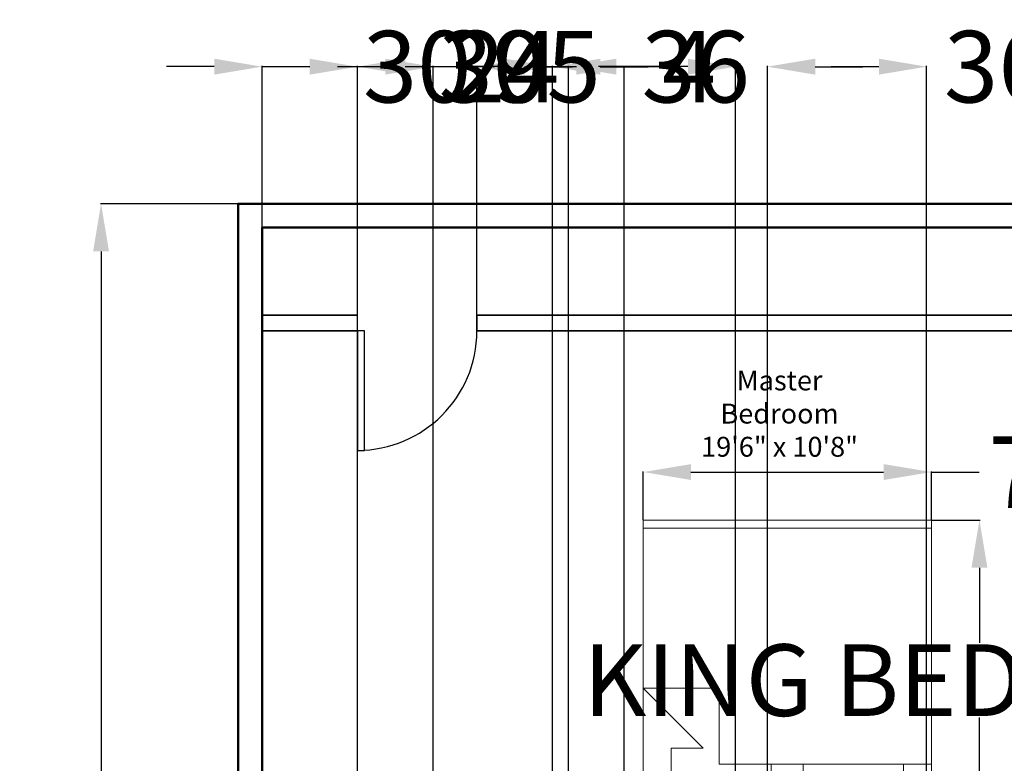
# Model space of a CAD drawing. Units: inches. Extents: x -230 to 384, y -962 to -183.
# Tile 5 of 6: x -156 to 91, y -370 to -183. Entities that reach past the tile are written whole.
import ezdxf

# ---------------------------------------------------------------- set-up
doc = ezdxf.new("R2010")
doc.units = ezdxf.units.IN
for name, color, linetype, lineweight in [('A-ANNO-DIMS', 2, 'Continuous', 18), ('A-AREA-IDEN', 7, 'Continuous', 18), ('A-DOOR', 3, 'Continuous', 25), ('Furniture', 2, 'Continuous', 18), ('Inner Wall', 5, 'Continuous', 35), ('Outer Wall', 1, 'Continuous', 50)]:
    doc.layers.add(name, color=color, linetype=linetype, lineweight=lineweight)
doc.styles.get("Standard").update_dxf_attribs({"font": 'arial.ttf'})
doc.dimstyles.get("Standard").update_dxf_attribs({"dimtxt": 18, "dimasz": 12, "dimexe": 0.18, "dimexo": 0.0625, "dimgap": 0.09, "dimtad": 0, "dimtih": 1, "dimtoh": 1, "dimdec": 0, "dimzin": 0, "dimdsep": 46, "dimlunit": 3, "dimtxsty": 'Standard', "dimcen": 0.09, "dimadec": 0, "dimazin": 0, "dimtfac": 1, "dimtdec": 0, "dimtofl": 0, "dimtmove": 0, "dimatfit": 3, "dimfxl": 1, "dimtolj": 1, "dimtzin": 0, "dimarcsym": 0})

# ---------------------------------------------------------------- blocks, each defined once
blk = doc.blocks.new('*U3')
for p, q in [((-30, 0), (-30, -4)), ((0, 0), (0, -4))]:
    blk.add_line(p, q)
blk.add_lwpolyline([(0, 0), (0, 30), (-1.75, 30), (-1.75, 0)], close=True)
blk.add_arc((0, 0), 30, 90, 180)
blk = doc.blocks.new('KING-00')
for p, q in [((-0.8967, -0.947), (-0.8967, 0.8818)), ((0.6019, 0.8818), (0.6019, -0.4644)), ((1.0337, -0.947), (1.0337, 0.8818)), ((0.6019, 0.704), (0.8813, 0.704)), ((0.8813, 0.069), (0.8813, 0.704)), ((0.6019, 0.069), (0.8813, 0.069)), ((0.8813, -0.1342), (0.6019, -0.1342)), ((0.8813, -0.7692), (0.8813, -0.1342)), ((0.1193, -0.4644), (0.1193, -0.947)), ((0.6019, -0.4644), (0.1193, -0.4644)), ((0.1193, -0.947), (0.5003, -0.566)), ((0.5003, -0.7692), (0.5003, -0.566)), ((0.5003, -0.7692), (0.8813, -0.7692))]:
    blk.add_line(p, q)
blk.add_lwpolyline([(-0.9475, -0.947), (-0.9475, 0.8818), (1.0845, 0.8818), (1.0845, -0.947)], close=True)
blk = doc.blocks.new('*D16')
at = {"layer": 'A-ANNO-DIMS', "color": 0, "lineweight": -2, "transparency": 16777216}
for p, q in [((72.67, -308.78), (84.86, -308.78)), ((84.68, -320.78), (84.68, -339.62)), ((84.68, -377.25), (84.68, -358.42)), ((72.67, -389.25), (84.86, -389.25))]:
    blk.add_line(p, q, dxfattribs=at)
at = {"layer": 'A-ANNO-DIMS', "color": 0, "transparency": 16777216}
for points in [[(82.68, -320.78), (86.68, -320.78), (84.68, -308.78)], [(82.68, -377.25), (86.68, -377.25), (84.68, -389.25)]]:
    blk.add_solid(points, dxfattribs=at)
at = {"layer": 'Defpoints', "color": 0, "transparency": 16777216}
for p in [(72.61, -308.78), (72.61, -389.25), (84.68, -389.25)]:
    blk.add_point(p, dxfattribs=at)
at = {"layer": 'A-ANNO-DIMS', "color": 0, "transparency": 16777216, "insert": (84.68, -349.02), "char_height": 18, "attachment_point": 5}
blk.add_mtext('\\A1;KING BED 80 TYP.', dxfattribs=at)
blk = doc.blocks.new('*D17')
at = {"layer": 'A-ANNO-DIMS', "color": 0, "lineweight": -2, "transparency": 16777216}
for p, q in [((0.19, -308.72), (0.19, -296.53)), ((12.19, -296.71), (60.61, -296.71)), ((72.61, -308.72), (72.61, -296.53)), ((72.61, -296.71), (84.61, -296.71))]:
    blk.add_line(p, q, dxfattribs=at)
at = {"layer": 'A-ANNO-DIMS', "color": 0, "transparency": 16777216}
for points in [[(12.19, -294.71), (12.19, -298.71), (0.19, -296.71)], [(60.61, -294.71), (60.61, -298.71), (72.61, -296.71)]]:
    blk.add_solid(points, dxfattribs=at)
at = {"layer": 'Defpoints', "color": 0, "transparency": 16777216}
for p in [(72.61, -296.71), (0.19, -308.78), (72.61, -308.78)]:
    blk.add_point(p, dxfattribs=at)
at = {"layer": 'A-ANNO-DIMS', "color": 0, "transparency": 16777216, "insert": (128.44, -296.71), "char_height": 18, "attachment_point": 5}
blk.add_mtext('\\A1;72 TYP.', dxfattribs=at)
blk = doc.blocks.new('*D33')
at = {"layer": 'A-ANNO-DIMS', "color": 0, "lineweight": -2, "transparency": 16777216}
for p, q in [((-101.66, -229.25), (-136.23, -229.25)), ((-136.05, -241.25), (-136.05, -562.97)), ((-136.05, -903.25), (-136.05, -581.53)), ((-101.66, -915.25), (-136.23, -915.25))]:
    blk.add_line(p, q, dxfattribs=at)
at = {"layer": 'A-ANNO-DIMS', "color": 0, "transparency": 16777216}
for points in [[(-138.05, -241.25), (-134.05, -241.25), (-136.05, -229.25)], [(-138.05, -903.25), (-134.05, -903.25), (-136.05, -915.25)]]:
    blk.add_solid(points, dxfattribs=at)
at = {"layer": 'Defpoints', "color": 0, "transparency": 16777216}
for p in [(-101.6, -229.25), (-136.05, -915.25), (-101.6, -915.25)]:
    blk.add_point(p, dxfattribs=at)
at = {"layer": 'A-ANNO-DIMS', "color": 0, "transparency": 16777216, "insert": (-136.05, -572.25), "char_height": 18, "attachment_point": 5}
blk.add_mtext('\\A1;686', dxfattribs=at)
blk = doc.blocks.new('*D35')
at = {"layer": 'A-ANNO-DIMS', "color": 0, "lineweight": -2, "transparency": 16777216}
for p, q in [((-107.6, -194.8), (-119.6, -194.8)), ((-95.6, -257.19), (-95.6, -194.62)), ((-71.6, -257.19), (-71.6, -194.62)), ((-59.6, -194.8), (-47.6, -194.8))]:
    blk.add_line(p, q, dxfattribs=at)
at = {"layer": 'A-ANNO-DIMS', "color": 0, "transparency": 16777216}
for points in [[(-107.6, -192.8), (-107.6, -196.8), (-95.6, -194.8)], [(-59.6, -192.8), (-59.6, -196.8), (-71.6, -194.8)]]:
    blk.add_solid(points, dxfattribs=at)
at = {"layer": 'Defpoints', "color": 0, "transparency": 16777216}
for p in [(-71.6, -194.8), (-95.6, -257.25), (-71.6, -257.25)]:
    blk.add_point(p, dxfattribs=at)
at = {"layer": 'A-ANNO-DIMS', "color": 0, "transparency": 16777216, "insert": (-34.5, -194.8), "char_height": 18, "attachment_point": 5}
blk.add_mtext('\\A1;24', dxfattribs=at)
blk = doc.blocks.new('*D36')
at = {"layer": 'A-ANNO-DIMS', "color": 0, "lineweight": -2, "transparency": 16777216}
for p, q in [((-83.60199, -194.80445), (-95.60199, -194.80445)), ((-71.60199, -257.19195), (-71.60199, -194.62445)), ((-41.60199, -257.19195), (-41.60199, -194.62445)), ((-29.60199, -194.80445), (-17.60199, -194.80445))]:
    blk.add_line(p, q, dxfattribs=at)
at = {"layer": 'A-ANNO-DIMS', "color": 0, "transparency": 16777216}
for points in [[(-83.60199, -192.80445), (-83.60199, -196.80445), (-71.60199, -194.80445)], [(-29.60199, -192.80445), (-29.60199, -196.80445), (-41.60199, -194.80445)]]:
    blk.add_solid(points, dxfattribs=at)
at = {"layer": 'Defpoints', "color": 0, "transparency": 16777216}
for p in [(-41.60199, -194.80445), (-71.60199, -257.25445), (-41.60199, -257.25445)]:
    blk.add_point(p, dxfattribs=at)
at = {"layer": 'A-ANNO-DIMS', "color": 0, "transparency": 16777216, "insert": (-56.60199, -194.80445), "char_height": 18, "attachment_point": 5}
blk.add_mtext('\\A1;30', dxfattribs=at)
blk = doc.blocks.new('*D42')
at = {"layer": 'A-ANNO-DIMS', "color": 0, "lineweight": -2, "transparency": 16777216}
for p, q in [((-64.60199, -194.80445), (-76.60199, -194.80445)), ((-52.60199, -389.19195), (-52.60199, -194.62445)), ((-22.60199, -389.19195), (-22.60199, -194.62445)), ((-10.60199, -194.80445), (1.39801, -194.80445))]:
    blk.add_line(p, q, dxfattribs=at)
at = {"layer": 'A-ANNO-DIMS', "color": 0, "transparency": 16777216}
for points in [[(-64.60199, -192.80445), (-64.60199, -196.80445), (-52.60199, -194.80445)], [(-10.60199, -192.80445), (-10.60199, -196.80445), (-22.60199, -194.80445)]]:
    blk.add_solid(points, dxfattribs=at)
at = {"layer": 'Defpoints', "color": 0, "transparency": 16777216}
for p in [(-22.60199, -194.80445), (-52.60199, -389.25445), (-22.60199, -389.25445)]:
    blk.add_point(p, dxfattribs=at)
at = {"layer": 'A-ANNO-DIMS', "color": 0, "transparency": 16777216, "insert": (-37.60199, -194.80445), "char_height": 18, "attachment_point": 5}
blk.add_mtext('\\A1;30', dxfattribs=at)
blk = doc.blocks.new('*D43')
at = {"layer": 'A-ANNO-DIMS', "color": 0, "lineweight": -2, "transparency": 16777216}
for p, q in [((-71.6, -510.19), (-71.6, -194.62)), ((-59.6, -194.8), (-37.15, -194.8)), ((11.4, -194.8), (-11.05, -194.8)), ((23.4, -510.19), (23.4, -194.62))]:
    blk.add_line(p, q, dxfattribs=at)
at = {"layer": 'A-ANNO-DIMS', "color": 0, "transparency": 16777216}
for points in [[(-59.6, -192.8), (-59.6, -196.8), (-71.6, -194.8)], [(11.4, -192.8), (11.4, -196.8), (23.4, -194.8)]]:
    blk.add_solid(points, dxfattribs=at)
at = {"layer": 'Defpoints', "color": 0, "transparency": 16777216}
for p in [(23.4, -194.8), (-71.6, -510.25), (23.4, -510.25)]:
    blk.add_point(p, dxfattribs=at)
at = {"layer": 'A-ANNO-DIMS', "color": 0, "transparency": 16777216, "insert": (-24.1, -194.8), "char_height": 18, "attachment_point": 5}
blk.add_mtext('\\A1;95', dxfattribs=at)
blk = doc.blocks.new('*D45')
at = {"layer": 'A-ANNO-DIMS', "color": 0, "lineweight": -2, "transparency": 16777216}
for p, q in [((-34.6, -194.8), (-46.6, -194.8)), ((-22.6, -389.19), (-22.6, -194.62)), ((-18.6, -393.19), (-18.6, -194.62)), ((-6.6, -194.8), (5.4, -194.8))]:
    blk.add_line(p, q, dxfattribs=at)
at = {"layer": 'A-ANNO-DIMS', "color": 0, "transparency": 16777216}
for points in [[(-34.6, -192.8), (-34.6, -196.8), (-22.6, -194.8)], [(-6.6, -192.8), (-6.6, -196.8), (-18.6, -194.8)]]:
    blk.add_solid(points, dxfattribs=at)
at = {"layer": 'Defpoints', "color": 0, "transparency": 16777216}
for p in [(-18.6, -194.8), (-22.6, -389.25), (-18.6, -393.25)]:
    blk.add_point(p, dxfattribs=at)
at = {"layer": 'A-ANNO-DIMS', "color": 0, "transparency": 16777216, "insert": (11.71, -194.8), "char_height": 18, "attachment_point": 5}
blk.add_mtext('\\A1;4', dxfattribs=at)
blk = doc.blocks.new('*D50')
at = {"layer": 'A-ANNO-DIMS', "color": 0, "lineweight": -2, "transparency": 16777216}
for p, q in [((59.39801, -194.80445), (47.39801, -194.80445)), ((71.39801, -534.19195), (71.39801, -194.62445)), ((107.39801, -534.19195), (107.39801, -194.62445)), ((119.39801, -194.80445), (131.39801, -194.80445))]:
    blk.add_line(p, q, dxfattribs=at)
at = {"layer": 'A-ANNO-DIMS', "color": 0, "transparency": 16777216}
for points in [[(59.39801, -192.80445), (59.39801, -196.80445), (71.39801, -194.80445)], [(119.39801, -192.80445), (119.39801, -196.80445), (107.39801, -194.80445)]]:
    blk.add_solid(points, dxfattribs=at)
at = {"layer": 'Defpoints', "color": 0, "transparency": 16777216}
for p in [(107.39801, -194.80445), (71.39801, -534.25445), (107.39801, -534.25445)]:
    blk.add_point(p, dxfattribs=at)
at = {"layer": 'A-ANNO-DIMS', "color": 0, "transparency": 16777216, "insert": (89.39801, -194.80445), "char_height": 18, "attachment_point": 5}
blk.add_mtext('\\A1;36', dxfattribs=at)
blk = doc.blocks.new('*D51')
at = {"layer": 'A-ANNO-DIMS', "color": 0, "lineweight": -2, "transparency": 16777216}
for p, q in [((-16.60199, -194.80445), (-28.60199, -194.80445)), ((-4.60199, -875.19195), (-4.60199, -194.62445)), ((31.39801, -875.19195), (31.39801, -194.62445)), ((43.39801, -194.80445), (55.39801, -194.80445))]:
    blk.add_line(p, q, dxfattribs=at)
at = {"layer": 'A-ANNO-DIMS', "color": 0, "transparency": 16777216}
for points in [[(-16.60199, -192.80445), (-16.60199, -196.80445), (-4.60199, -194.80445)], [(43.39801, -192.80445), (43.39801, -196.80445), (31.39801, -194.80445)]]:
    blk.add_solid(points, dxfattribs=at)
at = {"layer": 'Defpoints', "color": 0, "transparency": 16777216}
for p in [(31.39801, -194.80445), (-4.60199, -875.25445), (31.39801, -875.25445)]:
    blk.add_point(p, dxfattribs=at)
at = {"layer": 'A-ANNO-DIMS', "color": 0, "transparency": 16777216, "insert": (13.39801, -194.80445), "char_height": 18, "attachment_point": 5}
blk.add_mtext('\\A1;36', dxfattribs=at)

msp = doc.modelspace()

# ---------------------------------------------------------------- linework, layer by layer
at = {"layer": 'Furniture'}
msp.add_lwpolyline([(-71.6, -389.25), (-95.6, -389.25), (-95.6, -261.25), (-71.6, -261.25)], close=True, dxfattribs=at)
at = {"layer": 'Inner Wall'}
for p, q in [((-95.6, -257.25), (-71.6, -257.25)), ((-41.6, -261.25), (-41.6, -257.25)), ((-41.6, -257.25), (147.4, -257.25)), ((-95.6, -261.25), (-71.6, -261.25)), ((-41.6, -261.25), (137.4, -261.25))]:
    msp.add_line(p, q, dxfattribs=at)
at = {"layer": 'Outer Wall'}
for p, q in [((-95.6, -909.25), (-95.6, -235.25)), ((-95.6, -235.25), (266.4, -235.25))]:
    msp.add_line(p, q, dxfattribs=at)
msp.add_lwpolyline([(272.4, -915.25), (-101.6, -915.25), (-101.6, -229.25), (272.4, -229.25)], close=True, dxfattribs=at)

# ---------------------------------------------------------------- block references
at = {"layer": 'A-DOOR', "rotation": 180}
msp.add_blockref('*U3', (-71.6, -261.25), dxfattribs=at)
at = {"layer": 'Furniture', "xscale": 39.60249106241186, "yscale": 39.60249106241186, "zscale": 39.60249106241186, "rotation": 270}
msp.add_blockref('KING-00', (37.69, -346.31), dxfattribs=at)

# ---------------------------------------------------------------- texts
at = {"layer": 'A-AREA-IDEN', "insert": (59, -271.18), "char_height": 5, "attachment_point": 3}
msp.add_mtext_dynamic_manual_height_columns('\\pxqc;{\\fTimes New Roman|b0|i0|c0|p18;Master Bedroom\\P19\'6" x 10\'8"}', width=49.1019, gutter_width=12.5, heights=[0], dxfattribs=at)

# ---------------------------------------------------------------- dimensions: what is measured, and where the dimension line sits
at = {"layer": 'A-ANNO-DIMS'}
for base, p1, p2, picture, middle in [((-71.6, -194.8), (-95.6, -257.25), (-71.6, -257.25), '*D35', (-34.5, -194.8)), ((-41.6, -194.8), (-71.6, -257.25), (-41.6, -257.25), '*D36', (-56.6, -194.8)), ((-22.6, -194.8), (-52.6, -389.25), (-22.6, -389.25), '*D42', (-37.6, -194.8)), ((23.4, -194.8), (-71.6, -510.25), (23.4, -510.25), '*D43', (-24.1, -194.8)), ((-18.6, -194.8), (-22.6, -389.25), (-18.6, -393.25), '*D45', (11.71, -194.8)), ((31.4, -194.8), (-4.6, -875.25), (31.4, -875.25), '*D51', (13.4, -194.8)), ((107.4, -194.8), (71.4, -534.25), (107.4, -534.25), '*D50', (89.4, -194.8))]:
    dim = msp.add_linear_dim(base=base, p1=p1, p2=p2, dimstyle='Standard', override={"dimdec": 0, "dimlfac": 1, "dimrnd": 0, "dimzin": 0, "dimdsep": 46, "dimlunit": 2}, dxfattribs=at)
    dim.commit()
    dim.dimension.update_dxf_attribs({"geometry": picture, "text_midpoint": middle})
dim = msp.add_linear_dim(base=(-136.05, -915.25), p1=(-101.6, -229.25), p2=(-101.6, -915.25), angle=90, dimstyle='Standard', override={"dimdec": 0, "dimlfac": 1, "dimrnd": 0, "dimzin": 0, "dimdsep": 46, "dimlunit": 2}, dxfattribs=at)
dim.commit()
dim.dimension.update_dxf_attribs({"geometry": '*D33', "text_midpoint": (-136.05, -572.25)})
dim = msp.add_linear_dim(base=(72.61, -296.71), p1=(0.19, -308.78), p2=(72.61, -308.78), text='<> TYP.', dimstyle='Standard', override={"dimdec": 0, "dimlfac": 1, "dimrnd": 0, "dimzin": 0, "dimdsep": 46, "dimlunit": 2}, dxfattribs=at)
dim.commit()
dim.dimension.update_dxf_attribs({"geometry": '*D17', "text_midpoint": (128.44, -296.71)})
dim = msp.add_linear_dim(base=(84.68, -389.25), p1=(72.61, -308.78), p2=(72.61, -389.25), angle=270, text='KING BED <> TYP.', dimstyle='Standard', override={"dimdec": 0, "dimlfac": 1, "dimrnd": 0, "dimzin": 0, "dimdsep": 46, "dimlunit": 2}, dxfattribs=at)
dim.commit()
dim.dimension.update_dxf_attribs({"geometry": '*D16', "text_midpoint": (84.68, -349.02)})

doc.saveas('drawing.dxf')
